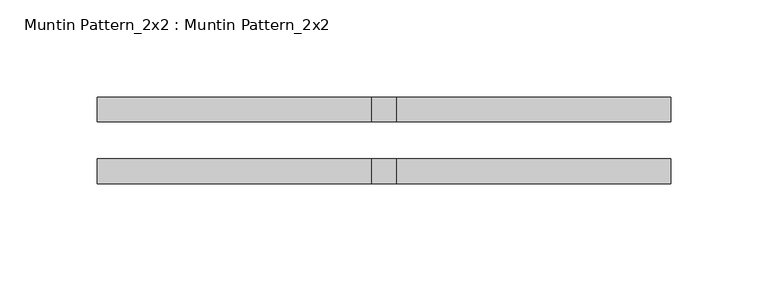
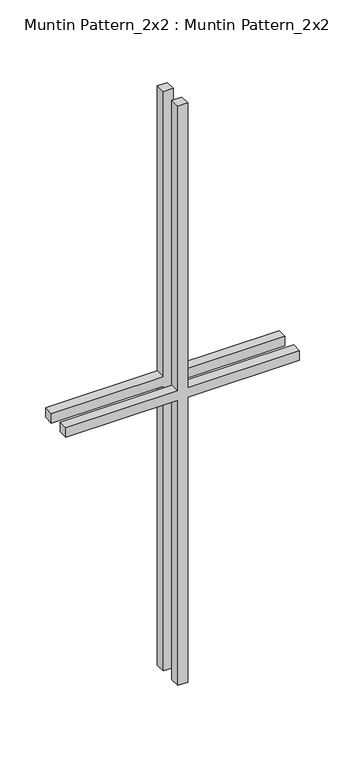
"""IFC4 building model written with IfcOpenShell, lengths in millimetres: proxy geometry, Muntin Pattern_2x2 : Muntin Pattern_2x2."""

from ifc_helpers import new_model, si_unit, frame, origin, place, context, project, spatial, polyline, outline, extrude, source, transform, mapped, element, save


def muntin_pattern_2x2_muntin_pattern_2x2_3e0ecaf2(model_context):
    return source(origin(), model_context, "Body", "SweptSolid", [
        extrude(outline(polyline([(393.7, -6.35), (393.7, -147.6375), (381.0, -147.6375), (381.0, -6.35), (0.0, -6.35), (0.0, 6.35), (381.0, 6.35), (381.0, 147.6375), (393.7, 147.6375), (393.7, 6.35), (774.7, 6.35), (774.7, -6.35), (393.7, -6.35)])), frame((0.0, -22.225, 0.0), z_axis=(0.0, 1.0, 0.0), x_axis=(0.0, 0.0, 1.0)), (0.0, 0.0, 1.0), 12.7),
        extrude(outline(polyline([(393.7, -6.35), (393.7, -147.6375), (381.0, -147.6375), (381.0, -6.35), (0.0, -6.35), (0.0, 6.35), (381.0, 6.35), (381.0, 147.6375), (393.7, 147.6375), (393.7, 6.35), (774.7, 6.35), (774.7, -6.35), (393.7, -6.35)])), frame((0.0, 9.525, 0.0), z_axis=(0.0, 1.0, 0.0), x_axis=(0.0, 0.0, 1.0)), (0.0, 0.0, 1.0), 12.7),
    ])


if __name__ == "__main__":
    model = new_model("IFC4")
    model_context = context("Model", 3, world=origin())
    ifc_project = project(units=[si_unit("LENGTHUNIT", "METRE", prefix="MILLI")], contexts=[model_context])
    site = spatial("IfcSite", under=ifc_project)
    building = spatial("IfcBuilding", under=site)
    placement = place(None, origin())
    muntin_pattern_2x2_muntin_pattern_2x2_shape = muntin_pattern_2x2_muntin_pattern_2x2_3e0ecaf2(model_context)
    element("IfcBuildingElementProxy", 1, Name="Muntin Pattern_2x2 : Muntin Pattern_2x2", ObjectType="Muntin Pattern_2x2 : Muntin Pattern_2x2", at=placement, inside=building, context=model_context, shape_type="MappedRepresentation", body=[
        mapped(muntin_pattern_2x2_muntin_pattern_2x2_shape, transform((0.0, 0.0, 0.0), x_axis=(1.0, 0.0, 0.0), y_axis=(0.0, 1.0, 0.0), z_axis=(0.0, 0.0, 1.0))),
    ])
    save(model, "model.ifc")

# Revit data of these elements
# Type "Muntin Pattern_2x2 : Muntin Pattern_2x2"
#   Width [instance default] = 4' - 0"
#   Thickness = 0' - 0 1/2"
#   Height [instance default] = 4' - 0"
#   Distance = 0' - 0 3/4"
#   Interior Material [instance default] = none
#   Exterior Material [instance default] = none
#   Default Elevation = 0
# Element 1 (IfcBuildingElementProxy, "Muntin Pattern_2x2 : Muntin Pattern_2x2")
#   Width = 0' - 11 5/8"
#   Height = 2' - 6 1/2"
#   Interior Material = Wood - Stained
#   Exterior Material = Clad - White
#   Materials on its faces: "Clad - White", "Wood - Stained"
# Materials
#   "Clad - White": class "Wood", colour RGB 30 30 30, transparency 0, Cost = 0
#   "Wood - Stained": class "Wood", colour RGB 224 178 126, transparency 0, Cost = 0
